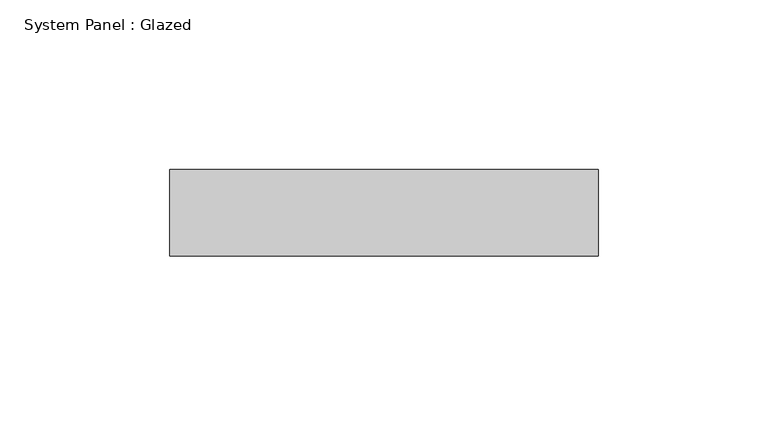
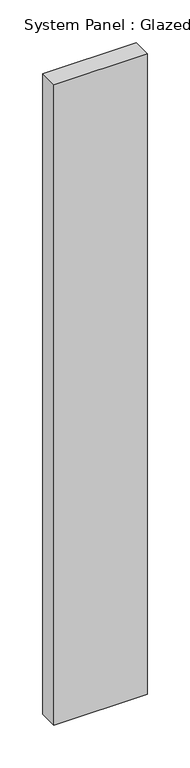
"""IFC4 building model written with IfcOpenShell, lengths in millimetres: plate geometry, System Panel : Glazed."""

from ifc_helpers import new_model, si_unit, origin, origin_with_axes, place, context, project, spatial, polyline, outline, extrude, source, transform, mapped, element, save


def system_panel_glazed_d0e8c3c7(model_context):
    return source(origin(), model_context, "Body", "SweptSolid", [
        extrude(outline(polyline([(63.0705981, 19.05), (-63.0705981, 19.05), (-63.0705981, 44.45), (63.0705981, 44.45), (63.0705981, 19.05)])), origin_with_axes(), (0.0, 0.0, 1.0), 914.4),
    ])


if __name__ == "__main__":
    model = new_model("IFC4")
    model_context = context("Model", 3, world=origin())
    ifc_project = project(units=[si_unit("LENGTHUNIT", "METRE", prefix="MILLI")], contexts=[model_context])
    site = spatial("IfcSite", under=ifc_project)
    building = spatial("IfcBuilding", under=site)
    placement = place(None, origin())
    system_panel_glazed_shape = system_panel_glazed_d0e8c3c7(model_context)
    element("IfcPlate", 1, ObjectType="System Panel : Glazed", at=placement, inside=building, context=model_context, shape_type="MappedRepresentation", body=[
        mapped(system_panel_glazed_shape, transform((0.0, 0.0, 0.0), x_axis=(1.0, 0.0, 0.0), y_axis=(0.0, 1.0, 0.0), z_axis=(0.0, 0.0, 1.0))),
    ])
    save(model, "model.ifc")

# Revit data of these elements
# Type "System Panel : Glazed"
#   Construction Type Id = "GSP4R"
#   Analytic Construction = "1/8 in Pilkington single glazing"
#   Visual Light Transmittance = 0.9
#   Solar Heat Gain Coefficient = 0.86
#   Heat Transfer Coefficient (U) = 6.7069 W/(m²·K)
# Element 1 (IfcPlate, "System Panel : Glazed")
#   Materials on its faces: "Glass"
# Materials
#   "Glass": class "Glass", colour RGB 0 128 192, transparency 0.75, Description = "Soda Lime Glass", Cost = 0
